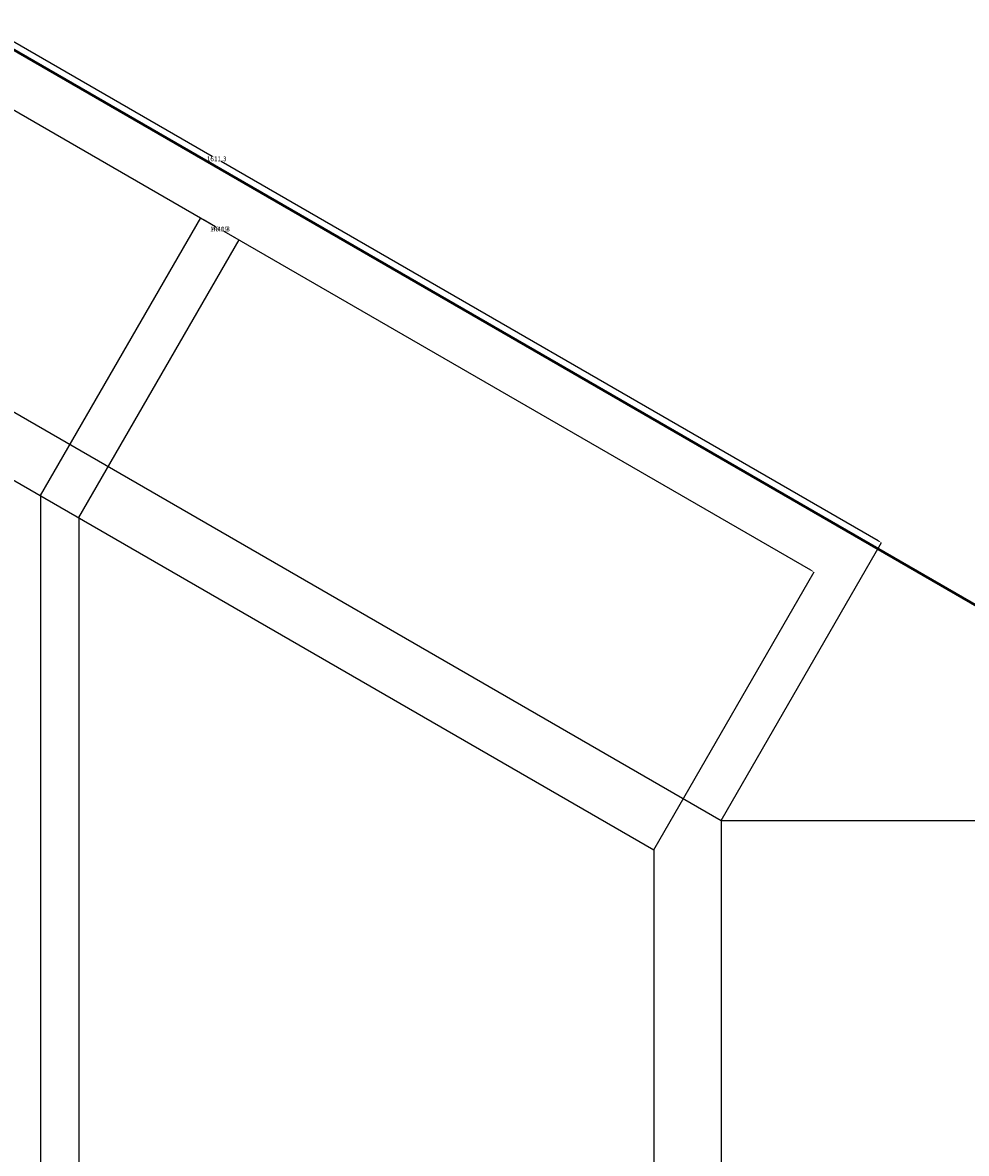
# Model space of a CAD drawing. Units: metres. Extents: x -2391 to 4922, y -635 to 4845.
# Tile 33 of 37: x 2158 to 3149, y 2425 to 3611. Entities that reach past the tile are written whole.
import ezdxf

# ---------------------------------------------------------------- set-up
doc = ezdxf.new("R2010")
doc.units = ezdxf.units.M
doc.header["$MEASUREMENT"] = 0
for name, color, linetype, lineweight in [('A-ANNO-DIMS', 2, 'Continuous', 18), ('A-GLAZ', 4, 'Continuous', 25), ('A-WALL', 7, 'Continuous', 50)]:
    doc.layers.add(name, color=color, linetype=linetype, lineweight=lineweight)
doc.styles.get("Standard").update_dxf_attribs({"font": 'arial.ttf'})
doc.dimstyles.get("Standard").update_dxf_attribs({"dimtxt": 5, "dimasz": 4, "dimexe": 0.18, "dimexo": 0.0625, "dimgap": 0.09, "dimtad": 0, "dimtih": 1, "dimtoh": 1, "dimdec": 0, "dimzin": 0, "dimdsep": 46, "dimtxsty": 'Standard', "dimcen": 0.09, "dimadec": 0, "dimazin": 0, "dimtfac": 1, "dimtdec": 0, "dimtofl": 0, "dimtmove": 0, "dimatfit": 3, "dimfxl": 1, "dimtolj": 1, "dimtzin": 0, "dimarcsym": 0})

# ---------------------------------------------------------------- blocks, each defined once
blk = doc.blocks.new('*D8')
at = {"layer": 'A-ANNO-DIMS', "color": 0, "lineweight": -2, "transparency": 16777216}
for p, q in [((-2047.3, 3005.2), (-2047.3, -631.4)), ((4577.8, 2350.2), (4577.8, -631.4)), ((-2043.3, -631.2), (1257.6, -631.2)), ((4573.8, -631.2), (1272.8, -631.2))]:
    blk.add_line(p, q, dxfattribs=at)
at = {"layer": 'A-ANNO-DIMS', "color": 0, "transparency": 16777216}
for points in [[(-2043.3, -630.6), (-2043.3, -631.9), (-2047.3, -631.2)], [(4573.8, -630.6), (4573.8, -631.9), (4577.8, -631.2)]]:
    blk.add_solid(points, dxfattribs=at)
at = {"layer": 'Defpoints', "color": 0, "transparency": 16777216}
for p in [(-2047.3, 3005.3), (4577.8, 2350.3), (4577.8, -631.2)]:
    blk.add_point(p, dxfattribs=at)
at = {"layer": 'A-ANNO-DIMS', "color": 0, "transparency": 16777216, "insert": (1265.2, -631.2), "char_height": 5, "attachment_point": 5}
blk.add_mtext('\\A1;6625', dxfattribs=at)
blk = doc.blocks.new('*D12')
at = {"layer": 'A-ANNO-DIMS', "color": 0, "lineweight": -2, "transparency": 16777216}
for p, q in [((1496.1, 3579.7), (1664.4, 3871.2)), ((1667.7, 3869), (2357.4, 3470.9)), ((3056.2, 3067.4), (2366.6, 3465.6)), ((2891.5, 2774), (3059.8, 3065.6))]:
    blk.add_line(p, q, dxfattribs=at)
at = {"layer": 'A-ANNO-DIMS', "color": 0, "transparency": 16777216}
for points in [[(1668.1, 3869.6), (1667.4, 3868.5), (1664.3, 3871)], [(3056.6, 3068), (3055.9, 3066.8), (3059.7, 3065.4)]]:
    blk.add_solid(points, dxfattribs=at)
at = {"layer": 'Defpoints', "color": 0, "transparency": 16777216}
for p in [(1496, 3579.6), (3059.7, 3065.4), (2891.4, 2774)]:
    blk.add_point(p, dxfattribs=at)
at = {"layer": 'A-ANNO-DIMS', "color": 0, "transparency": 16777216, "insert": (2362, 3468.2), "char_height": 5, "attachment_point": 5}
blk.add_mtext('\\A1;1611.3', dxfattribs=at)
blk = doc.blocks.new('*D13')
at = {"layer": 'A-ANNO-DIMS', "color": 0, "lineweight": -2, "transparency": 16777216}
for p, q in [((2891.5, 2774), (3228.1, 2774)), ((3227.9, 2770), (3227.9, 2318)), ((3227.9, 1860.8), (3227.9, 2312.8)), ((2891.5, 1856.8), (3228.1, 1856.8))]:
    blk.add_line(p, q, dxfattribs=at)
at = {"layer": 'A-ANNO-DIMS', "color": 0, "transparency": 16777216}
for points in [[(3227.3, 2770), (3228.6, 2770), (3227.9, 2774)], [(3227.3, 1860.8), (3228.6, 1860.8), (3227.9, 1856.8)]]:
    blk.add_solid(points, dxfattribs=at)
at = {"layer": 'Defpoints', "color": 0, "transparency": 16777216}
for p in [(2891.4, 2774), (2891.4, 1856.8), (3227.9, 1856.8)]:
    blk.add_point(p, dxfattribs=at)
at = {"layer": 'A-ANNO-DIMS', "color": 0, "transparency": 16777216, "insert": (3227.9, 2315.4), "char_height": 5, "attachment_point": 5}
blk.add_mtext('\\A1;917.2', dxfattribs=at)
blk = doc.blocks.new('*D14')
at = {"layer": 'A-ANNO-DIMS', "color": 0, "lineweight": -2, "transparency": 16777216}
for p, q in [((1573.6, 3463.3), (1741.9, 3754.8)), ((1745.2, 3752.7), (2360.9, 3397.3)), ((2985.7, 3036.5), (2370, 3392)), ((2820.9, 2743.2), (2989.2, 3034.7))]:
    blk.add_line(p, q, dxfattribs=at)
at = {"layer": 'A-ANNO-DIMS', "color": 0, "transparency": 16777216}
for points in [[(1745.6, 3753.3), (1744.9, 3752.1), (1741.8, 3754.7)], [(2986, 3037.1), (2985.3, 3036), (2989.1, 3034.5)]]:
    blk.add_solid(points, dxfattribs=at)
at = {"layer": 'Defpoints', "color": 0, "transparency": 16777216}
for p in [(1573.5, 3463.3), (2989.1, 3034.5), (2820.9, 2743.1)]:
    blk.add_point(p, dxfattribs=at)
at = {"layer": 'A-ANNO-DIMS', "color": 0, "transparency": 16777216, "insert": (2365.5, 3394.6), "char_height": 5, "attachment_point": 5}
blk.add_mtext('\\A1;1440.3', dxfattribs=at)
blk = doc.blocks.new('*D16')
at = {"layer": 'A-ANNO-DIMS', "color": 0, "lineweight": -2, "transparency": 16777216}
for p, q in [((2177.2, 3114.8), (2345.5, 3406.3)), ((2348.9, 3404.2), (2360.9, 3397.3)), ((2217.2, 3091.7), (2385.5, 3383.2)), ((2382, 3385.1), (2370, 3392))]:
    blk.add_line(p, q, dxfattribs=at)
at = {"layer": 'A-ANNO-DIMS', "color": 0, "transparency": 16777216}
for points in [[(2349.2, 3404.7), (2348.6, 3403.6), (2345.5, 3406.2)], [(2382.3, 3385.6), (2381.7, 3384.5), (2385.5, 3383.1)]]:
    blk.add_solid(points, dxfattribs=at)
at = {"layer": 'Defpoints', "color": 0, "transparency": 16777216}
for p in [(2385.5, 3383.1), (2177.2, 3114.7), (2217.2, 3091.7)]:
    blk.add_point(p, dxfattribs=at)
at = {"layer": 'A-ANNO-DIMS', "color": 0, "transparency": 16777216, "insert": (2365.5, 3394.6), "char_height": 5, "attachment_point": 5}
blk.add_mtext('\\A1;46.19', dxfattribs=at)

msp = doc.modelspace()

# ---------------------------------------------------------------- linework, layer by layer
at = {"layer": 'A-GLAZ'}
for p, q in [((1496.0309, 3579.6156), (2891.4324, 2773.9801)), ((1573.5273, 3463.276), (2820.8768, 2743.1184)), ((2177.2021, 3114.7443), (2177.2021, 2329.8889)), ((2217.2021, 3091.6502), (2217.2021, 2306.7949)), ((2891.4324, 2773.9801), (2891.4324, 1856.8211)), ((2820.8768, 2743.1184), (2820.8768, 1958.2631))]:
    msp.add_line(p, q, dxfattribs=at)
at = {"layer": 'A-WALL'}
msp.add_line((550.7419, 4505.2763), (3607.8116, 2740.2763), dxfattribs=at)

# ---------------------------------------------------------------- dimensions: what is measured, and where the dimension line sits
at = {"layer": 'A-ANNO-DIMS'}
for base, p1, p2, angle, override, picture, middle in [((3059.6824, 3065.3977), (1496.0309, 3579.6156), (2891.4324, 2773.9801), 330, {"dimdec": 1, "dimlfac": 1, "dimrnd": 0, "dimzin": 0, "dimdsep": 46, "dimlunit": 2}, '*D12', (2361.9817, 3468.2154)), ((2989.1268, 3034.536), (1573.5273, 3463.276), (2820.8768, 2743.1184), 330, {"dimdec": 1, "dimlfac": 1, "dimrnd": 0, "dimzin": 0, "dimdsep": 46, "dimlunit": 2}, '*D14', (2365.4521, 3394.6148)), ((2385.4521, 3383.0678), (2177.2021, 3114.7443), (2217.2021, 3091.6502), 330, {"dimdec": 2, "dimlfac": 1, "dimrnd": 0, "dimzin": 0, "dimdsep": 46, "dimlunit": 2}, '*D16', (2365.4521, 3394.6148)), ((3227.9324, 1856.8211), (2891.4324, 2773.9801), (2891.4324, 1856.8211), 270, {"dimdec": 1, "dimlfac": 1, "dimrnd": 0, "dimzin": 0, "dimdsep": 46, "dimlunit": 2}, '*D13', (3227.9324, 2315.4006))]:
    dim = msp.add_linear_dim(base=base, p1=p1, p2=p2, angle=angle, dimstyle='Standard', override=override, dxfattribs=at)
    dim.commit()
    dim.dimension.update_dxf_attribs({"geometry": picture, "text_midpoint": middle})
dim = msp.add_linear_dim(base=(4577.76, -631.2237), p1=(-2047.3343, 3005.2763), p2=(4577.76, 2350.2763), dimstyle='Standard', override={"dimdec": 0, "dimlfac": 1, "dimrnd": 0, "dimzin": 0, "dimdsep": 46, "dimlunit": 2}, dxfattribs=at)
dim.commit()
dim.dimension.update_dxf_attribs({"geometry": '*D8', "text_midpoint": (1265.2128, -631.2237)})

doc.saveas('drawing.dxf')
